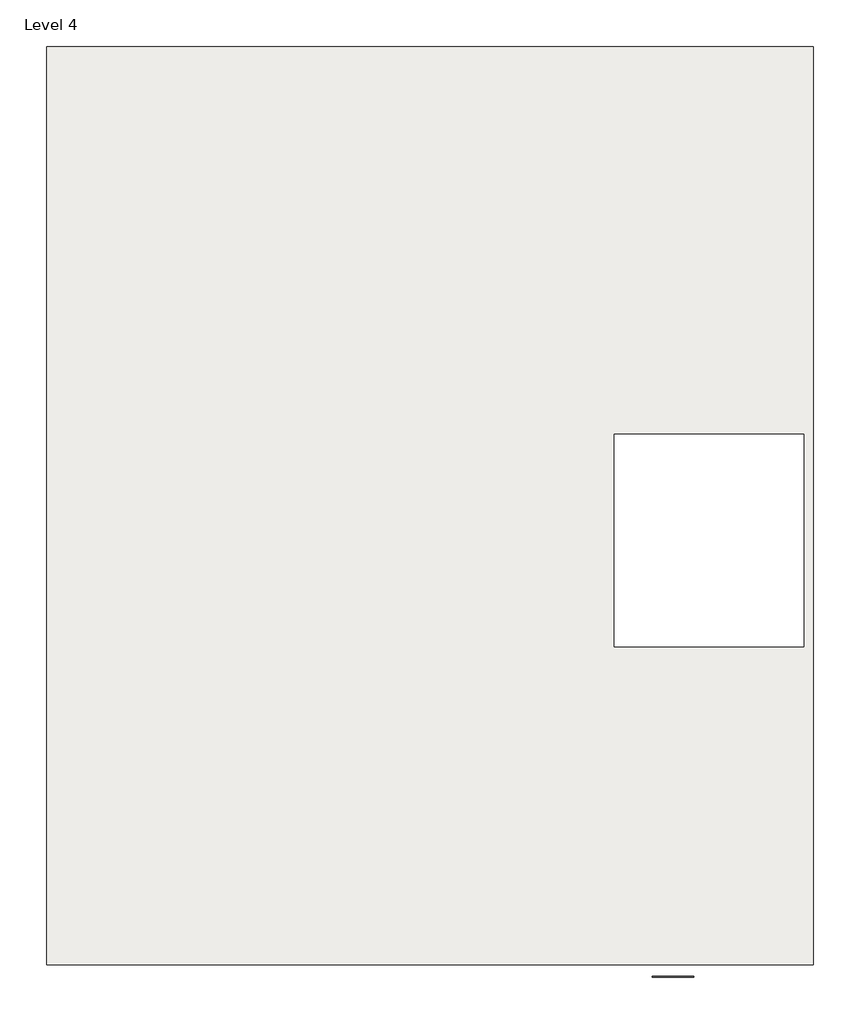
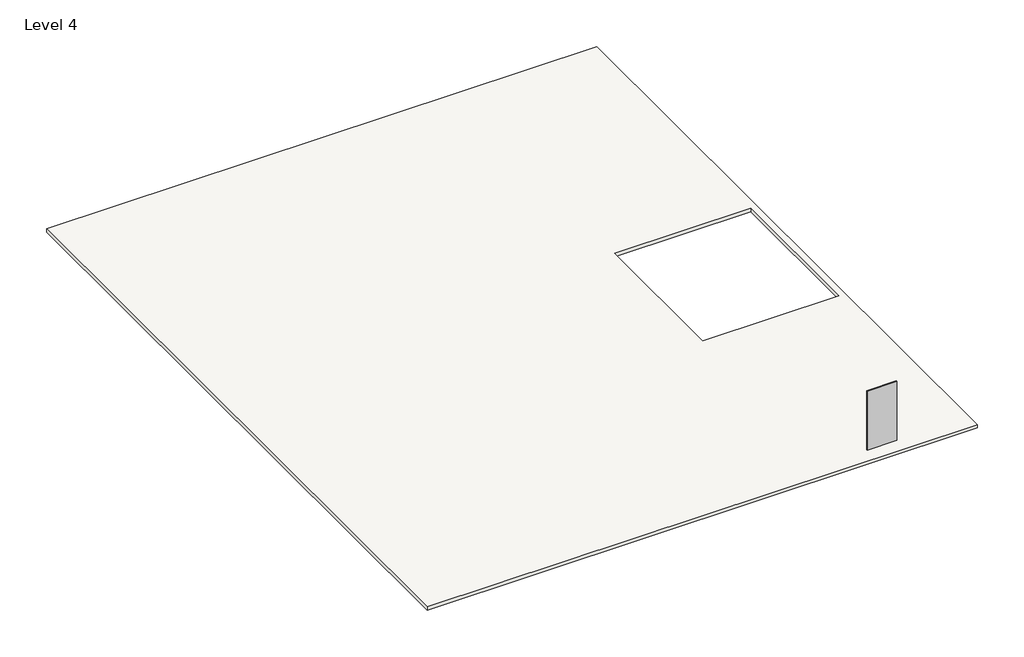
# One storey: 1 plate, 1 slab.
"""IFC4 building model written with IfcOpenShell, lengths in millimetres."""

from ifc_helpers import new_model, si_unit, frame, origin, place, context, project, spatial, polyline, outline, extrude, transform, mapped, element, save
from components import system_panel_glazed_1b7191b4

model = new_model("IFC4")

# Units and contexts
model_context = context("Model", 3, world=origin())
ifc_project = project(units=[si_unit("LENGTHUNIT", "METRE", prefix="MILLI")], contexts=[model_context])

# Site, building, storey
site = spatial("IfcSite", under=ifc_project)
building = spatial("IfcBuilding", under=site)
storey = spatial("IfcBuildingStorey", under=building, Name="Level 4", Elevation=7162.8)

# Plate
placement = place(None, origin())
system_panel_glazed_shape = system_panel_glazed_1b7191b4(model_context)
element("IfcPlate", 1, ObjectType="System Panel : Glazed", at=placement, inside=storey, context=model_context, shape_type="MappedRepresentation", body=[
    mapped(system_panel_glazed_shape, transform((5161.5954883, -15325.4077095, 7696.2), x_axis=(1.0, 0.0, 0.0), y_axis=(0.0, 1.0, 0.0), z_axis=(0.0, 0.0, 1.0))),
])

# Slab
element("IfcSlab", 2, ObjectType="Generic - 4\"", at=placement, inside=storey, context=model_context, shape_type="SweptSolid", body=[
    extrude(outline(polyline([(-7454.7186876, -15050.3330955), (-7454.7186876, 3440.8669045), (7988.4813124, 3440.8669045), (7988.4813124, -15050.3330955), (-7454.7186876, -15050.3330955)]), holes=[polyline([(7797.9813124, -4367.7173694), (3981.0893946, -4367.7173694), (3981.0893946, -8648.1976656), (7797.9813124, -8648.1976656), (7797.9813124, -4367.7173694)])]), frame((0.0, 0.0, 7061.2), z_axis=(0.0, 0.0, 1.0), x_axis=(1.0, 0.0, 0.0)), (0.0, 0.0, 1.0), 101.6),
])

save(model, "model.ifc")

# Revit data of these elements
# Type "System Panel : Glazed"
#   Construction Type Id = "GSP4R"
#   Analytic Construction = "1/8 in Pilkington single glazing"
#   Visual Light Transmittance = 0.9
#   Solar Heat Gain Coefficient = 0.86
#   Heat Transfer Coefficient (U) = 1.18115 BTU/(h·ft²·°F)
#   Define Thermal Properties by = 1
# Type "Generic - 4\""
#   Assembly Code = "B1010"
#   Function = 0
#   Layers, outside or top first: 0' - 4" no material (function 1)
# Element 1 (IfcPlate, "System Panel : Glazed")
#   Phase Created = New Construction
#   Materials on its faces: "Glass"
# Element 2 (IfcSlab, "Generic - 4\"")
#   built-in parameter 1001955 = -1.5708 (stored number, unit not read)
#   Height Offset From Level = 0' - 0"
#   Phase Created = New Construction
#   Materials on its faces: "Default Floor", "floor"
# Materials
#   "Glass": class "Glass", colour RGB 0 128 192, transparency 0.75, Description = "Soda Lime Glass", Cost = 0
#   "Default Floor": colour RGB 128 128 128, transparency 0, Cost = 0
#   "floor": class "Generic", colour RGB 255 207 159, transparency 0, Cost = 0
